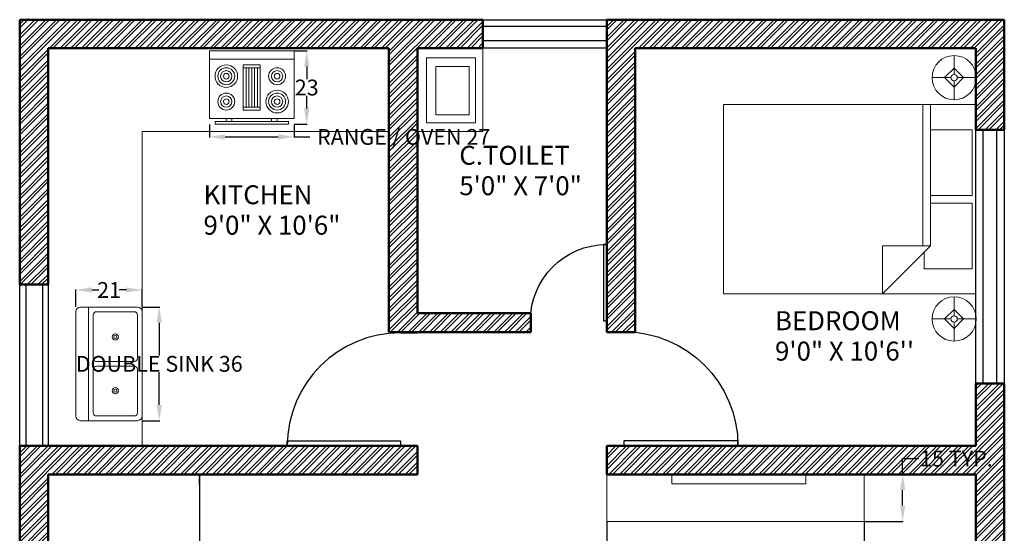
# Model space of a CAD drawing. Units: inches. Extents: x 0 to 822, y 0 to 962.
# Tile 2 of 3: x 24 to 336, y 799 to 962. Entities that reach past the tile are written whole.
import ezdxf

# ---------------------------------------------------------------- set-up
doc = ezdxf.new("R2010")
doc.units = ezdxf.units.IN
doc.header["$MEASUREMENT"] = 0
for name, color, linetype, lineweight in [('A-ANNO-DIMS', 2, 'Continuous', 18), ('A-AREA-IDEN', 7, 'Continuous', 25), ('A-DOOR', 4, 'Continuous', 25), ('A-FLOR-CASE', 5, 'Continuous', 18), ('A-FLOR-FIXT', 8, 'Continuous', 18), ('A-FLOR-STRS', 3, 'Continuous', 25), ('A-FURN', 9, 'Continuous', 18), ('A-GLAZ', 4, 'Continuous', 25), ('A-WALL', 7, 'Continuous', 50), ('A-WALL-PATT', 8, 'Continuous', 13)]:
    doc.layers.add(name, color=color, linetype=linetype, lineweight=lineweight)
doc.styles.get("Standard").update_dxf_attribs({"font": 'arial.ttf'})
doc.dimstyles.get("Standard").update_dxf_attribs({"dimtxt": 5, "dimasz": 5, "dimexe": 0.18, "dimexo": 0.0625, "dimgap": 0.09, "dimtad": 0, "dimtih": 1, "dimtoh": 1, "dimdec": 1, "dimzin": 0, "dimdsep": 46, "dimlunit": 4, "dimtxsty": 'Standard', "dimcen": 0.09, "dimadec": 0, "dimazin": 0, "dimtfac": 1, "dimtdec": 1, "dimtofl": 0, "dimtmove": 0, "dimatfit": 3, "dimfxl": 1, "dimtolj": 1, "dimtzin": 0, "dimarcsym": 0})

# ---------------------------------------------------------------- blocks, each defined once
blk = doc.blocks.new('*U2')
for p, q in [((0, 0), (0, -6)), ((40, 0), (40, -6))]:
    blk.add_line(p, q)
blk.add_lwpolyline([(0, 0), (0, 40), (1.75, 40), (1.75, 0)], close=True)
blk.add_arc((0, 0), 40, 0, 90)
blk = doc.blocks.new('Range-Oven - 30 in top')
for p, q in [((0, -3), (30, -3)), ((12, -6), (18, -6)), ((13, -20), (13, -6)), ((14, -6), (14, -20)), ((15, -20), (15, -6)), ((16, -6), (16, -20)), ((17, -20), (17, -6)), ((18, -20), (12, -20)), ((6, -24), (6, -25)), ((8, -25), (8, -24)), ((22, -25), (22, -24)), ((24, -24), (24, -25))]:
    blk.add_line(p, q)
for points in [[(0, -24), (0, 0), (30, 0), (30, -24)], [(12, -21), (12, -5), (18, -5), (18, -21)], [(2, -26), (2, -25), (28, -25), (28, -26)]]:
    blk.add_lwpolyline(points, close=True)
for centre, radius in [((6, -9), 4), ((6, -9), 3), ((24, -9), 3), ((6, -9), 2), ((6, -9), 1), ((24, -9), 2), ((24, -9), 1), ((6, -18), 3), ((6, -18), 2), ((6, -18), 1), ((24, -18), 4), ((24, -18), 3), ((24, -18), 2), ((24, -18), 1)]:
    blk.add_circle(centre, radius)
blk = doc.blocks.new('Sink-double - 36 in top')
for p, q in [((-18, -4), (18, -4)), ((-0.75, -18.5), (-0.75, -6.5)), ((0.75, -6.5), (0.75, -18.5))]:
    blk.add_line(p, q)
for points in [[(-16.5, 0), (16.5, 0)], [(-18, -19.5), (-18, -1.5)], [(18, -1.5), (18, -19.5)], [(-15.5, -5.5), (-1.75, -5.5)], [(1.75, -5.5), (15.5, -5.5)], [(-16.5, -18.5), (-16.5, -6.5)], [(16.5, -6.5), (16.5, -18.5)], [(16.5, -21), (-16.5, -21)], [(-1.75, -19.5), (-15.5, -19.5)], [(15.5, -19.5), (1.75, -19.5)]]:
    blk.add_lwpolyline(points)
for centre, radius in [((-8.5, -12.5), 1), ((-8.5, -12.5), 0.5), ((8.5, -12.5), 1), ((8.5, -12.5), 0.5)]:
    blk.add_circle(centre, radius)
for centre, radius, start, end in [((-16.5, -1.5), 1.5, 90, 180), ((16.5, -1.5), 1.5, 0, 90), ((-15.5, -6.5), 1, 90, 180), ((-1.75, -6.5), 1, 0, 90), ((1.75, -6.5), 1, 90, 180), ((15.5, -6.5), 1, 0, 90), ((-15.5, -18.5), 1, 180, 270), ((-1.75, -18.5), 1, 270, 0), ((1.75, -18.5), 1, 180, 270), ((15.5, -18.5), 1, 270, 0), ((-16.5, -19.5), 1.5, 180, 270), ((16.5, -19.5), 1.5, 270, 0)]:
    blk.add_arc(centre, radius, start, end)
blk = doc.blocks.new('Bed - Queen')
for p, q in [((0, -80.00003), (0, 0)), ((0, 0), (59.99999, 0)), ((59.99999, 0), (59.99999, -80.00003)), ((7.99999, -1.2), (28.79998, -1.2)), ((7.99999, -14.4), (7.99999, -1.2)), ((28.79998, -1.2), (28.79998, -14.4)), ((31.19999, -1.2), (51.99999, -1.2)), ((31.19999, -14.4), (31.19999, -1.2)), ((51.99999, -1.2), (51.99999, -16.4)), ((0, -14.4), (44.8, -14.4)), ((59.99999, -29.6), (44.8, -14.4)), ((44.8, -14.4), (44.8, -29.6)), ((44.8, -16.8), (0, -16.8)), ((51.99999, -16.4), (46.79936, -16.4)), ((44.8, -29.6), (59.99999, -29.6)), ((59.99999, -80.00003), (0, -80.00003))]:
    blk.add_line(p, q)
blk = doc.blocks.new('Lamp - Table')
for p, q in [((0, 7), (0, 1)), ((-1, 0), (-7, 0)), ((0, 3), (-3, 0)), ((-3, 0), (0, -3)), ((3, 0), (0, 3)), ((0, -3), (3, 0)), ((1, 0), (7, 0)), ((0, -1), (0, -7))]:
    blk.add_line(p, q)
for radius in [7, 1]:
    blk.add_circle((0, 0), radius)
blk = doc.blocks.new('TV-UNIT')
for points in [[(0, 14.91), (81.55, 14.91), (81.55, 0), (0, 0)], [(20.69, 14.91), (63.1, 14.91), (63.1, 11.87), (20.69, 11.87)]]:
    blk.add_lwpolyline(points, close=True)
blk = doc.blocks.new('*D27')
at = {"layer": 'A-ANNO-DIMS', "color": 0, "lineweight": -2, "transparency": 16777216}
for p, q in [((209.73, 802.98), (209.73, 790.63)), ((291.28, 802.98), (291.28, 790.63)), ((214.73, 790.81), (223.63, 790.81)), ((286.28, 790.81), (277.38, 790.81))]:
    blk.add_line(p, q, dxfattribs=at)
at = {"layer": 'A-ANNO-DIMS', "color": 0, "transparency": 16777216}
for points in [[(214.73, 791.64), (214.73, 789.97), (209.73, 790.81)], [(286.28, 791.64), (286.28, 789.97), (291.28, 790.81)]]:
    blk.add_solid(points, dxfattribs=at)
at = {"layer": 'Defpoints', "color": 0, "transparency": 16777216}
for p in [(209.73, 803.04), (291.28, 803.04), (291.28, 790.81)]:
    blk.add_point(p, dxfattribs=at)
at = {"layer": 'A-ANNO-DIMS', "color": 0, "transparency": 16777216, "insert": (250.5, 790.81), "char_height": 5, "attachment_point": 5}
blk.add_mtext('\\A1;TV UNIT 82 TYP.', dxfattribs=at)
blk = doc.blocks.new('*D28')
at = {"layer": 'A-ANNO-DIMS', "color": 0, "lineweight": -2, "transparency": 16777216}
for p, q in [((303.51, 817.95), (303.51, 822.95)), ((303.51, 822.95), (308.51, 822.95)), ((291.34, 817.95), (303.69, 817.95)), ((303.51, 808.04), (303.51, 812.95)), ((291.34, 803.04), (303.69, 803.04))]:
    blk.add_line(p, q, dxfattribs=at)
at = {"layer": 'A-ANNO-DIMS', "color": 0, "transparency": 16777216}
for points in [[(302.68, 812.95), (304.34, 812.95), (303.51, 817.95)], [(302.68, 808.04), (304.34, 808.04), (303.51, 803.04)]]:
    blk.add_solid(points, dxfattribs=at)
at = {"layer": 'Defpoints', "color": 0, "transparency": 16777216}
for p in [(291.28, 817.95), (303.51, 817.95), (291.28, 803.04)]:
    blk.add_point(p, dxfattribs=at)
at = {"layer": 'A-ANNO-DIMS', "color": 0, "transparency": 16777216, "insert": (320.53, 822.95), "char_height": 5, "attachment_point": 5}
blk.add_mtext('\\A1;15 TYP.', dxfattribs=at)
blk = doc.blocks.new('*D37')
at = {"layer": 'A-ANNO-DIMS', "color": 0, "lineweight": -2, "transparency": 16777216}
for p, q in [((83.83, 928.78), (83.83, 924.64)), ((110.66, 928.78), (110.66, 924.64)), ((88.83, 924.82), (105.66, 924.82)), ((110.66, 924.82), (115.66, 924.82))]:
    blk.add_line(p, q, dxfattribs=at)
at = {"layer": 'A-ANNO-DIMS', "color": 0, "transparency": 16777216}
for points in [[(88.83, 925.65), (88.83, 923.98), (83.83, 924.82)], [(105.66, 925.65), (105.66, 923.98), (110.66, 924.82)]]:
    blk.add_solid(points, dxfattribs=at)
at = {"layer": 'Defpoints', "color": 0, "transparency": 16777216}
for p in [(83.83, 928.84), (110.66, 928.84), (110.66, 924.82)]:
    blk.add_point(p, dxfattribs=at)
at = {"layer": 'A-ANNO-DIMS', "color": 0, "transparency": 16777216, "insert": (145.4, 924.82), "char_height": 5, "attachment_point": 5}
blk.add_mtext('\\A1;RANGE / OVEN 27', dxfattribs=at)
blk = doc.blocks.new('*D38')
at = {"layer": 'A-ANNO-DIMS', "color": 0, "lineweight": -2, "transparency": 16777216}
for p, q in [((110.72, 952.1), (114.86, 952.1)), ((114.68, 947.1), (114.68, 943.11)), ((114.68, 933.84), (114.68, 937.82)), ((110.72, 928.84), (114.86, 928.84))]:
    blk.add_line(p, q, dxfattribs=at)
at = {"layer": 'A-ANNO-DIMS', "color": 0, "transparency": 16777216}
for points in [[(113.85, 947.1), (115.52, 947.1), (114.68, 952.1)], [(113.85, 933.84), (115.52, 933.84), (114.68, 928.84)]]:
    blk.add_solid(points, dxfattribs=at)
at = {"layer": 'Defpoints', "color": 0, "transparency": 16777216}
for p in [(110.66, 952.1), (114.68, 952.1), (110.66, 928.84)]:
    blk.add_point(p, dxfattribs=at)
at = {"layer": 'A-ANNO-DIMS', "color": 0, "transparency": 16777216, "insert": (114.68, 940.47), "char_height": 5, "attachment_point": 5}
blk.add_mtext('\\A1;23', dxfattribs=at)
blk = doc.blocks.new('*D39')
at = {"layer": 'A-ANNO-DIMS', "color": 0, "lineweight": -2, "transparency": 16777216}
for p, q in [((62.6, 870.95), (68.12, 870.95)), ((67.94, 865.95), (67.94, 855.63)), ((67.94, 839.95), (67.94, 850.27)), ((62.6, 834.95), (68.12, 834.95))]:
    blk.add_line(p, q, dxfattribs=at)
at = {"layer": 'A-ANNO-DIMS', "color": 0, "transparency": 16777216}
for points in [[(67.1, 865.95), (68.77, 865.95), (67.94, 870.95)], [(67.1, 839.95), (68.77, 839.95), (67.94, 834.95)]]:
    blk.add_solid(points, dxfattribs=at)
at = {"layer": 'Defpoints', "color": 0, "transparency": 16777216}
for p in [(62.54, 870.95), (67.94, 870.95), (62.54, 834.95)]:
    blk.add_point(p, dxfattribs=at)
at = {"layer": 'A-ANNO-DIMS', "color": 0, "transparency": 16777216, "insert": (67.94, 852.95), "char_height": 5, "attachment_point": 5}
blk.add_mtext('\\A1;DOUBLE SINK 36', dxfattribs=at)
blk = doc.blocks.new('*D40')
at = {"layer": 'A-ANNO-DIMS', "color": 0, "lineweight": -2, "transparency": 16777216}
for p, q in [((41.54, 871.01), (41.54, 876.53)), ((46.54, 876.35), (48.8, 876.35)), ((57.54, 876.35), (55.27, 876.35)), ((62.54, 871.01), (62.54, 876.53))]:
    blk.add_line(p, q, dxfattribs=at)
at = {"layer": 'A-ANNO-DIMS', "color": 0, "transparency": 16777216}
for points in [[(46.54, 877.18), (46.54, 875.52), (41.54, 876.35)], [(57.54, 877.18), (57.54, 875.52), (62.54, 876.35)]]:
    blk.add_solid(points, dxfattribs=at)
at = {"layer": 'Defpoints', "color": 0, "transparency": 16777216}
for p in [(41.54, 876.35), (41.54, 870.95), (62.54, 870.95)]:
    blk.add_point(p, dxfattribs=at)
at = {"layer": 'A-ANNO-DIMS', "color": 0, "transparency": 16777216, "insert": (52.04, 876.35), "char_height": 5, "attachment_point": 5}
blk.add_mtext('\\A1;21', dxfattribs=at)

msp = doc.modelspace()

# ---------------------------------------------------------------- hatches: boundary and pattern name
at = {"layer": 'A-WALL-PATT', "transparency": 33554641}
h = msp.add_hatch(dxfattribs=at)
h.set_pattern_fill('ANSI32', color=256, scale=6.4)
h.paths.add_polyline_path([(149.73, 826.95), (23.73, 826.95), (23.73, 547.95), (87.48, 547.95), (87.48, 556.95), (32.73, 556.95), (32.73, 676.95), (179.73, 676.95), (179.73, 685.95), (32.73, 685.95), (32.73, 817.95), (149.73, 817.95)])
h.paths.add_polyline_path([(224.73, 685.95), (215.73, 685.95), (215.73, 556.95), (168.56, 556.95), (168.56, 547.95), (224.73, 547.95), (224.73, 589.95), (278.73, 589.95), (278.73, 595.95), (224.73, 595.95)])
h.paths.add_polyline_path([(278.73, 685.95), (272.73, 685.95), (272.73, 631.95), (278.73, 631.95)])
h.paths.add_polyline_path([(335.73, 719.52), (326.73, 719.52), (326.73, 676.95), (326.73, 589.95), (326.73, 501.45), (335.73, 501.45)])
h.paths.add_polyline_path([(335.73, 846.75), (326.73, 846.75), (326.73, 826.95), (209.73, 826.95), (209.73, 817.95), (326.73, 817.95), (326.73, 770.62), (335.73, 770.62)])
h.paths.add_polyline_path([(218.73, 952.95), (326.73, 952.95), (326.73, 927.05), (335.73, 927.05), (335.73, 961.95), (209.73, 961.95), (209.73, 952.95), (209.73, 862.95), (218.73, 862.95)])
h.paths.add_polyline_path([(149.73, 952.95), (170.53, 952.95), (170.53, 961.95), (23.73, 961.95), (23.73, 878.05), (32.73, 878.05), (32.73, 952.95), (140.73, 952.95), (140.73, 862.95), (185.73, 862.95), (185.73, 868.95), (149.73, 868.95)])

# ---------------------------------------------------------------- linework, layer by layer
at = {"layer": 'A-FLOR-CASE'}
for p, q in [((170.53, 926.53), (170.53, 952.95)), ((62.54, 826.95), (62.54, 926.53)), ((62.54, 926.53), (140.73, 926.53)), ((149.73, 926.53), (170.53, 926.53))]:
    msp.add_line(p, q, dxfattribs=at)
at = {"layer": 'A-FLOR-FIXT'}
for points in [[(152.66, 949.87), (168.17, 949.87), (168.17, 929.31), (152.66, 929.31)], [(155.56, 947.1), (166.13, 947.1), (166.13, 931.86), (155.56, 931.86)]]:
    msp.add_lwpolyline(points, close=True, dxfattribs=at)
at = {"layer": 'A-FLOR-STRS'}
for p, q in [((80.73, 814.67), (80.73, 817.95)), ((80.73, 817.95), (80.73, 781.95))]:
    msp.add_line(p, q, dxfattribs=at)
at = {"layer": 'A-GLAZ'}
for points in [[(170.53, 961.95), (209.73, 961.95), (209.73, 952.95), (170.53, 952.95)], [(170.53, 959.91), (209.73, 959.91), (209.73, 955.21), (170.53, 955.21)], [(326.73, 927.05), (335.73, 927.05), (335.73, 846.75), (326.73, 846.75)], [(329, 927.05), (333.23, 927.05), (333.23, 846.75), (329, 846.75)], [(32.73, 826.95), (23.73, 826.95), (23.73, 878.05), (32.73, 878.05)], [(25.74, 878.05), (30.93, 878.05), (30.93, 826.95), (25.74, 826.95)]]:
    msp.add_lwpolyline(points, close=True, dxfattribs=at)
at = {"layer": 'A-WALL'}
for p, q in [((23.73, 961.95), (23.73, 878.05)), ((170.53, 961.95), (23.73, 961.95)), ((170.53, 961.95), (170.53, 952.95)), ((209.73, 961.95), (209.73, 862.95)), ((335.73, 961.95), (209.73, 961.95)), ((335.73, 961.95), (335.73, 927.05)), ((32.73, 952.95), (32.73, 878.05)), ((32.73, 952.95), (140.73, 952.95)), ((140.73, 952.95), (140.73, 862.95)), ((149.73, 952.95), (149.73, 868.95)), ((149.73, 952.95), (170.53, 952.95)), ((218.73, 952.95), (218.73, 862.95)), ((218.73, 952.95), (326.73, 952.95)), ((326.73, 952.95), (326.73, 927.05)), ((326.73, 927.05), (335.73, 927.05)), ((23.73, 878.05), (32.73, 878.05)), ((149.73, 868.95), (185.73, 868.95)), ((185.73, 862.95), (185.73, 868.95)), ((140.73, 862.95), (185.73, 862.95)), ((209.73, 862.95), (218.73, 862.95)), ((326.73, 846.75), (335.73, 846.75)), ((326.73, 846.75), (326.73, 826.95)), ((335.73, 846.75), (335.73, 770.62)), ((23.73, 826.95), (149.73, 826.95)), ((23.73, 826.95), (23.73, 547.95)), ((149.73, 826.95), (149.73, 817.95)), ((209.73, 826.95), (326.73, 826.95)), ((209.73, 826.95), (209.73, 817.95)), ((32.73, 817.95), (149.73, 817.95)), ((32.73, 817.95), (32.73, 685.95)), ((209.73, 817.95), (326.73, 817.95)), ((326.73, 817.95), (326.73, 770.62))]:
    msp.add_line(p, q, dxfattribs=at)

# ---------------------------------------------------------------- block references
at = {"layer": 'A-DOOR', "xscale": -0.6046779911153904, "yscale": 0.6046779911153904, "zscale": 0.6046779911153904}
msp.add_blockref('*U2', (209.73, 866.57), dxfattribs=at)
at = {"layer": 'A-DOOR'}
for p, xscale, yscale, zscale, rotation in [((144.35, 826.95), 0.895952054503976, 0.895952054503976, 0.895952054503976, 90), ((215.15, 826.95), -0.9042162645231613, 0.9042162645231613, 0.9042162645231613, 270)]:
    msp.add_blockref('*U2', p, dxfattribs=dict(at, xscale=xscale, yscale=yscale, zscale=zscale, rotation=rotation))
at = {"layer": 'A-FLOR-FIXT', "xscale": 0.8944271909999159, "yscale": 0.8944271909999159, "zscale": 0.8944271909999159}
msp.add_blockref('Range-Oven - 30 in top', (83.83, 952.1), dxfattribs=at)
at = {"layer": 'A-FLOR-FIXT', "rotation": 90}
msp.add_blockref('Sink-double - 36 in top', (41.54, 852.95), dxfattribs=at)
at = {"layer": 'A-FURN', "rotation": 270}
for name, p in [('Lamp - Table', (319.82, 943.59)), ('Bed - Queen', (326.73, 935.08)), ('Lamp - Table', (319.82, 867.16))]:
    msp.add_blockref(name, p, dxfattribs=at)
at = {"layer": 'A-FURN'}
msp.add_blockref('TV-UNIT', (209.73, 803.04), dxfattribs=at)

# ---------------------------------------------------------------- texts
at = {"layer": 'A-AREA-IDEN'}
for s, p in [('C.TOILET', (163.03, 916)), ('5\'0" X 7\'0" ', (163.03, 906.36)), ('KITCHEN', (81.98, 903.5)), ('9\'0" X 10\'6"', (81.98, 893.86)), ('BEDROOM', (263.07, 863.61)), ('9\'0" X 10\'6\'\'', (263.07, 853.98))]:
    msp.add_text(s, height=6, dxfattribs=at).set_placement(p)

# ---------------------------------------------------------------- dimensions: what is measured, and where the dimension line sits
at = {"layer": 'A-ANNO-DIMS'}
for base, p1, p2, angle, picture, middle in [((114.68, 952.1), (110.66, 928.84), (110.66, 952.1), 90, '*D38', (114.68, 940.47)), ((41.54, 876.35), (62.54, 870.95), (41.54, 870.95), 180, '*D40', (52.04, 876.35))]:
    dim = msp.add_linear_dim(base=base, p1=p1, p2=p2, angle=angle, dimstyle='Standard', override={"dimdec": 0, "dimrnd": 0, "dimzin": 0, "dimlunit": 2}, dxfattribs=at)
    dim.commit()
    dim.dimension.update_dxf_attribs({"geometry": picture, "text_midpoint": middle})
for base, p1, p2, text, picture, middle in [((110.66, 924.82), (83.83, 928.84), (110.66, 928.84), 'RANGE / OVEN <>', '*D37', (145.4, 924.82)), ((291.28, 790.81), (209.73, 803.04), (291.28, 803.04), 'TV UNIT <> TYP.', '*D27', (250.5, 790.81))]:
    dim = msp.add_linear_dim(base=base, p1=p1, p2=p2, text=text, dimstyle='Standard', override={"dimdec": 0, "dimrnd": 0, "dimzin": 0, "dimlunit": 2}, dxfattribs=at)
    dim.commit()
    dim.dimension.update_dxf_attribs({"geometry": picture, "text_midpoint": middle})
for base, p1, p2, text, picture, middle in [((67.94, 870.95), (62.54, 834.95), (62.54, 870.95), 'DOUBLE SINK <>', '*D39', (67.94, 852.95)), ((303.51, 817.95), (291.28, 803.04), (291.28, 817.95), '<> TYP.', '*D28', (320.53, 822.95))]:
    dim = msp.add_linear_dim(base=base, p1=p1, p2=p2, angle=90, text=text, dimstyle='Standard', override={"dimdec": 0, "dimrnd": 0, "dimzin": 0, "dimlunit": 2}, dxfattribs=at)
    dim.commit()
    dim.dimension.update_dxf_attribs({"geometry": picture, "text_midpoint": middle})

doc.saveas('drawing.dxf')
